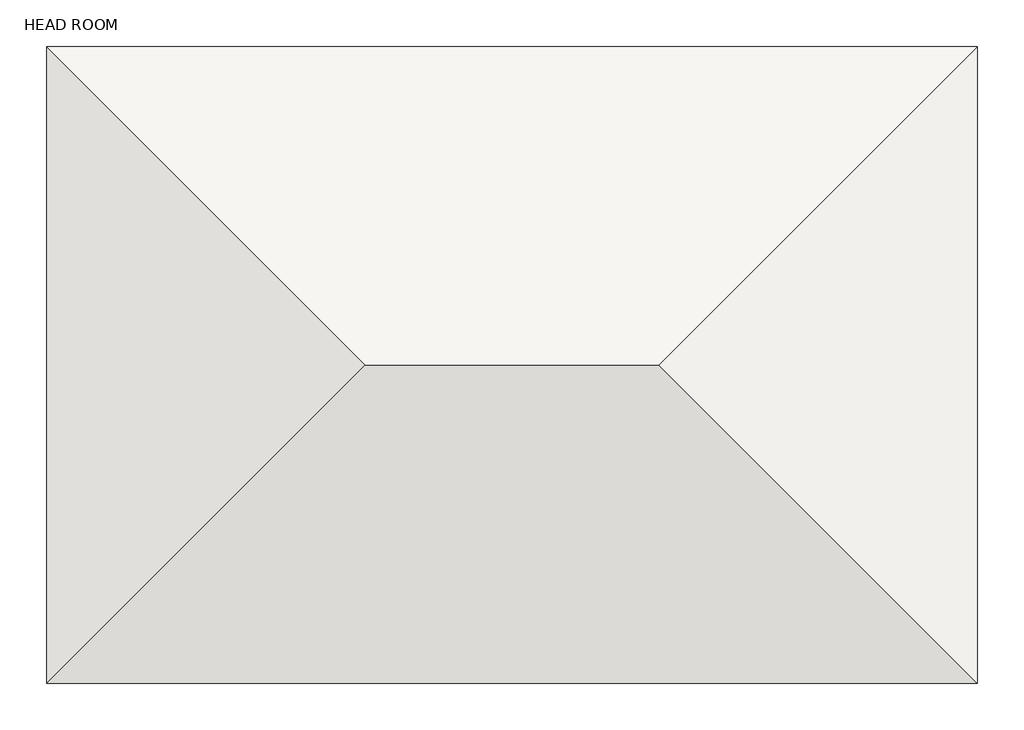
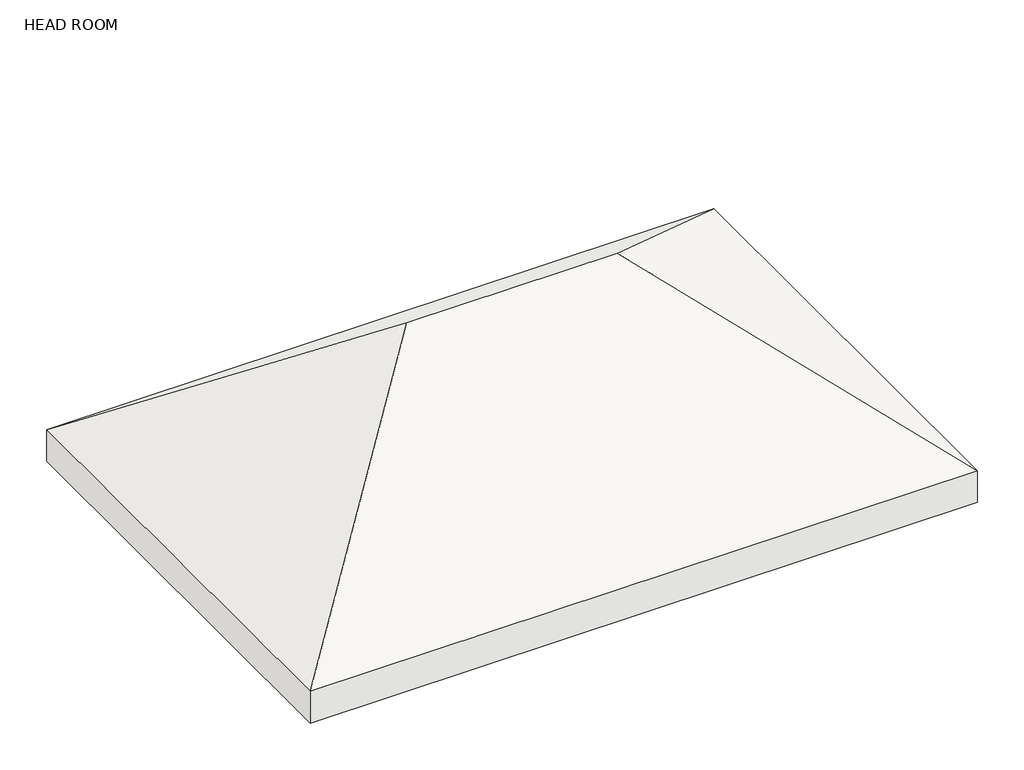
# One storey: 1 roof.
"""IFC4 building model written with IfcOpenShell, lengths in millimetres."""

from ifc_helpers import new_model, si_unit, origin, place, context, project, spatial, faceted_brep, element, save

model = new_model("IFC4")

# Units and contexts
model_context = context("Model", 3, world=origin())
ifc_project = project(units=[si_unit("LENGTHUNIT", "METRE", prefix="MILLI")], contexts=[model_context])

# Site, building, storey
site = spatial("IfcSite", under=ifc_project)
building = spatial("IfcBuilding", under=site)
storey = spatial("IfcBuildingStorey", under=building, Name="HEAD ROOM", Elevation=8534.4)

# Roof
placement = place(None, origin())
element("IfcRoof", 1, ObjectType="Generic - 12\"", at=placement, inside=storey, context=model_context, shape_type="Brep", body=[
    faceted_brep([(-11460.3436606, -2945.1024127, 9505.95), (-12755.7436606, -1649.7024127, 8534.4), (-8971.1436606, -1649.7024127, 8534.4), (-10266.5436606, -2945.1024127, 9505.95), (-8971.1436606, -4240.5024127, 8534.4), (-12755.7436606, -4240.5024127, 8534.4), (-12755.7436606, -1649.7024127, 8724.9), (-11460.3436606, -2945.1024127, 9696.45), (-10266.5436606, -2945.1024127, 9696.45), (-8971.1436606, -1649.7024127, 8724.9), (-8971.1436606, -4240.5024127, 8724.9), (-12755.7436606, -4240.5024127, 8724.9)], [[[0, 1, 2, 3]], [[4, 3, 2]], [[5, 0, 3, 4]], [[1, 0, 5]], [[6, 7, 8, 9]], [[10, 9, 8]], [[11, 10, 8, 7]], [[6, 11, 7]], [[5, 11, 6, 1]], [[4, 10, 11, 5]], [[2, 9, 10, 4]], [[1, 6, 9, 2]]]),
])

save(model, "model.ifc")

# Revit data of these elements
# Type "Generic - 12\""
#   Assembly Code = "B1020"
#   Layers, outside or top first: 0' - 6" "roof material" (function 1)
# Element 1 (IfcRoof, "Generic - 12\"")
#   built-in parameter 1001705 = 31.8125 (stored number, unit not read)
#   built-in parameter 1001710 = 33615
#   Phase Created = New Construction
#   Materials on its faces: "roof material"
# Materials
#   "roof material": class "Generic", colour RGB 120 120 120, transparency 0, Cost = 0
